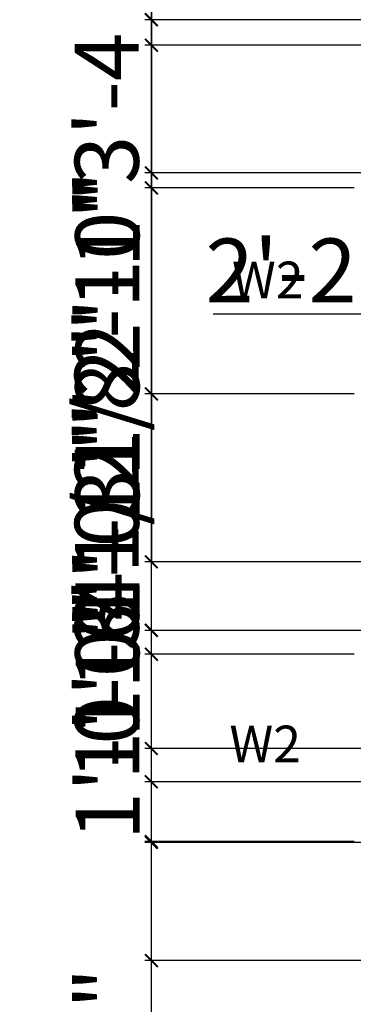
# Model space of a CAD drawing. Units: inches. Extents: x 1763 to 2368, y 1500 to 2097.
# Tile 5 of 24: x 1763 to 1828, y 1794 to 1986. Entities that reach past the tile are written whole.
import ezdxf

# ---------------------------------------------------------------- set-up
doc = ezdxf.new("R2010")
doc.units = ezdxf.units.IN
doc.layers.add('A-ANNO-DIMS', color=2, linetype='Continuous', lineweight=18)
doc.layers.add('A-ANNO-TEXT', color=7, linetype='Continuous', lineweight=18)
doc.styles.get("Standard").update_dxf_attribs({"font": 'arial.ttf'})
doc.dimstyles.new('ISO-25', dxfattribs={"dimtxt": 12.5, "dimasz": 2.5, "dimexe": 1.25, "dimexo": 0.625, "dimtad": 1, "dimdec": 0, "dimlunit": 4, "dimtxsty": 'Standard', "dimblk": 'ARCHTICK', "dimcen": 2.5, "dimclrd": 3, "dimclrt": 4, "dimadec": 0, "dimazin": 0, "dimtfac": 1, "dimtdec": 0, "dimtmove": 0, "dimatfit": 3, "dimfxl": 1, "dimarcsym": 0})

# ---------------------------------------------------------------- blocks, each defined once
blk = doc.blocks.new('_ArchTick')
at = {"color": 0, "linetype": 'ByBlock', "const_width": 0.15}
blk.add_lwpolyline([(-0.5, -0.5), (0.5, 0.5)], dxfattribs=at)
blk = doc.blocks.new('*D30')
at = {"layer": 'A-ANNO-DIMS', "color": 0, "lineweight": -2, "transparency": 16777216}
for p, q in [((1838.09, 1924.84), (1838.09, 1929.96)), ((1864.09, 1924.84), (1864.09, 1929.96))]:
    blk.add_line(p, q, dxfattribs=at)
at = {"layer": 'A-ANNO-DIMS', "color": 3, "lineweight": -2, "transparency": 16777216}
for p, q in [((1838.09, 1928.71), (1800.9, 1928.71)), ((1864.09, 1928.71), (1838.09, 1928.71))]:
    blk.add_line(p, q, dxfattribs=at)
at = {"layer": 'Defpoints', "color": 0, "transparency": 16777216}
for p in [(1838.09, 1928.71), (1838.09, 1924.21), (1864.09, 1924.21)]:
    blk.add_point(p, dxfattribs=at)
at = {"layer": 'A-ANNO-DIMS', "color": 3, "lineweight": -2, "transparency": 16777216, "xscale": 2.5, "yscale": 2.5, "zscale": 2.5, "rotation": 180}
blk.add_blockref('_ArchTick', (1838.09, 1928.71), dxfattribs=at)
at = {"layer": 'A-ANNO-DIMS', "color": 3, "lineweight": -2, "transparency": 16777216, "xscale": 2.5, "yscale": 2.5, "zscale": 2.5}
blk.add_blockref('_ArchTick', (1864.09, 1928.71), dxfattribs=at)
at = {"layer": 'A-ANNO-DIMS', "color": 4, "transparency": 16777216, "insert": (1818.25, 1935.61), "char_height": 12.5, "attachment_point": 5}
blk.add_mtext('2\'-2"', dxfattribs=at)
blk = doc.blocks.new('*D44')
at = {"layer": 'A-ANNO-DIMS', "color": 0, "lineweight": -2, "transparency": 16777216}
for p, q in [((1828.47, 2043.27), (1787.6, 2043.27)), ((1837.47, 1986.27), (1787.6, 1986.27))]:
    blk.add_line(p, q, dxfattribs=at)
at = {"layer": 'A-ANNO-DIMS', "color": 3, "lineweight": -2, "transparency": 16777216}
blk.add_line((1788.85, 2043.27), (1788.85, 1986.27), dxfattribs=at)
at = {"layer": 'Defpoints', "color": 0, "transparency": 16777216}
for p in [(1829.09, 2043.27), (1788.85, 1986.27), (1838.09, 1986.27)]:
    blk.add_point(p, dxfattribs=at)
at = {"layer": 'A-ANNO-DIMS', "color": 3, "lineweight": -2, "transparency": 16777216, "xscale": 2.5, "yscale": 2.5, "zscale": 2.5}
for p, rotation in [((1788.85, 2043.27), 90), ((1788.85, 1986.27), 270)]:
    blk.add_blockref('_ArchTick', p, dxfattribs=dict(at, rotation=rotation))
at = {"layer": 'A-ANNO-DIMS', "color": 4, "transparency": 16777216, "insert": (1781.85, 2014.77), "char_height": 12.5, "attachment_point": 5, "rotation": 90}
blk.add_mtext('4\'-9"', dxfattribs=at)
blk = doc.blocks.new('*D47')
at = {"layer": 'A-ANNO-DIMS', "color": 0, "lineweight": -2, "transparency": 16777216}
for p, q in [((1828.47, 1825.59), (1787.6, 1825.59)), ((1828.47, 1738.64), (1787.6, 1738.64))]:
    blk.add_line(p, q, dxfattribs=at)
at = {"layer": 'A-ANNO-DIMS', "color": 3, "lineweight": -2, "transparency": 16777216}
blk.add_line((1788.85, 1738.64), (1788.85, 1825.59), dxfattribs=at)
at = {"layer": 'Defpoints', "color": 0, "transparency": 16777216}
for p in [(1788.85, 1825.59), (1829.09, 1825.59), (1829.09, 1738.64)]:
    blk.add_point(p, dxfattribs=at)
at = {"layer": 'A-ANNO-DIMS', "color": 3, "lineweight": -2, "transparency": 16777216, "xscale": 2.5, "yscale": 2.5, "zscale": 2.5}
for p, rotation in [((1788.85, 1825.59), 90), ((1788.85, 1738.64), 270)]:
    blk.add_blockref('_ArchTick', p, dxfattribs=dict(at, rotation=rotation))
at = {"layer": 'A-ANNO-DIMS', "color": 4, "transparency": 16777216, "insert": (1781.84, 1782.12), "char_height": 12.5, "attachment_point": 5, "rotation": 90}
blk.add_mtext('7\'-3"', dxfattribs=at)
blk = doc.blocks.new('*D48')
at = {"layer": 'A-ANNO-DIMS', "color": 3, "lineweight": -2, "transparency": 16777216}
for p, q in [((1788.85, 1862.2), (1788.85, 1928.3)), ((1788.85, 1825.59), (1788.85, 1862.2))]:
    blk.add_line(p, q, dxfattribs=at)
at = {"layer": 'A-ANNO-DIMS', "color": 0, "lineweight": -2, "transparency": 16777216}
for p, q in [((1828.47, 1862.2), (1787.6, 1862.2)), ((1828.47, 1825.59), (1787.6, 1825.59))]:
    blk.add_line(p, q, dxfattribs=at)
at = {"layer": 'Defpoints', "color": 0, "transparency": 16777216}
for p in [(1788.85, 1862.2), (1829.09, 1862.2), (1829.09, 1825.59)]:
    blk.add_point(p, dxfattribs=at)
at = {"layer": 'A-ANNO-DIMS', "color": 3, "lineweight": -2, "transparency": 16777216, "xscale": 2.5, "yscale": 2.5, "zscale": 2.5}
for p, rotation in [((1788.85, 1862.2), 90), ((1788.85, 1825.59), 270)]:
    blk.add_blockref('_ArchTick', p, dxfattribs=dict(at, rotation=rotation))
at = {"layer": 'A-ANNO-DIMS', "color": 4, "transparency": 16777216, "insert": (1781.76, 1896.5), "char_height": 12.5, "attachment_point": 5, "rotation": 90}
blk.add_mtext('3\'-0 1/2"', dxfattribs=at)
blk = doc.blocks.new('*D49')
at = {"layer": 'A-ANNO-DIMS', "color": 0, "lineweight": -2, "transparency": 16777216}
for p, q in [((1828.47, 1913.1), (1787.6, 1913.1)), ((1828.47, 1862.2), (1787.6, 1862.2))]:
    blk.add_line(p, q, dxfattribs=at)
at = {"layer": 'A-ANNO-DIMS', "color": 3, "lineweight": -2, "transparency": 16777216}
blk.add_line((1788.85, 1862.2), (1788.85, 1913.1), dxfattribs=at)
at = {"layer": 'Defpoints', "color": 0, "transparency": 16777216}
for p in [(1788.85, 1913.1), (1829.09, 1913.1), (1829.09, 1862.2)]:
    blk.add_point(p, dxfattribs=at)
at = {"layer": 'A-ANNO-DIMS', "color": 3, "lineweight": -2, "transparency": 16777216, "xscale": 2.5, "yscale": 2.5, "zscale": 2.5}
for p, rotation in [((1788.85, 1913.1), 90), ((1788.85, 1862.2), 270)]:
    blk.add_blockref('_ArchTick', p, dxfattribs=dict(at, rotation=rotation))
at = {"layer": 'A-ANNO-DIMS', "color": 4, "transparency": 16777216, "insert": (1781.84, 1887.65), "char_height": 12.5, "attachment_point": 5, "rotation": 90}
blk.add_mtext('4\'-3"', dxfattribs=at)
blk = doc.blocks.new('*D50')
at = {"layer": 'A-ANNO-DIMS', "color": 3, "lineweight": -2, "transparency": 16777216}
for p, q in [((1788.85, 1953.39), (1788.85, 2019.48)), ((1788.85, 1913.1), (1788.85, 1953.39))]:
    blk.add_line(p, q, dxfattribs=at)
at = {"layer": 'A-ANNO-DIMS', "color": 0, "lineweight": -2, "transparency": 16777216}
for p, q in [((1828.47, 1953.39), (1787.6, 1953.39)), ((1828.47, 1913.1), (1787.6, 1913.1))]:
    blk.add_line(p, q, dxfattribs=at)
at = {"layer": 'Defpoints', "color": 0, "transparency": 16777216}
for p in [(1788.85, 1953.39), (1829.09, 1953.39), (1829.09, 1913.1)]:
    blk.add_point(p, dxfattribs=at)
at = {"layer": 'A-ANNO-DIMS', "color": 3, "lineweight": -2, "transparency": 16777216, "xscale": 2.5, "yscale": 2.5, "zscale": 2.5}
for p, rotation in [((1788.85, 1953.39), 90), ((1788.85, 1913.1), 270)]:
    blk.add_blockref('_ArchTick', p, dxfattribs=dict(at, rotation=rotation))
at = {"layer": 'A-ANNO-DIMS', "color": 4, "transparency": 16777216, "insert": (1781.76, 1987.69), "char_height": 12.5, "attachment_point": 5, "rotation": 90}
blk.add_mtext('3\'-4 1/2"', dxfattribs=at)
blk = doc.blocks.new('*D51')
at = {"layer": 'A-ANNO-DIMS', "color": 3, "lineweight": -2, "transparency": 16777216}
for p, q in [((1788.85, 1986.27), (1788.85, 2023.46)), ((1788.85, 1953.39), (1788.85, 1986.27))]:
    blk.add_line(p, q, dxfattribs=at)
at = {"layer": 'A-ANNO-DIMS', "color": 0, "lineweight": -2, "transparency": 16777216}
for p, q in [((1837.47, 1986.27), (1787.6, 1986.27)), ((1828.47, 1953.39), (1787.6, 1953.39))]:
    blk.add_line(p, q, dxfattribs=at)
at = {"layer": 'Defpoints', "color": 0, "transparency": 16777216}
for p in [(1788.85, 1986.27), (1838.09, 1986.27), (1829.09, 1953.39)]:
    blk.add_point(p, dxfattribs=at)
at = {"layer": 'A-ANNO-DIMS', "color": 3, "lineweight": -2, "transparency": 16777216, "xscale": 2.5, "yscale": 2.5, "zscale": 2.5}
for p, rotation in [((1788.85, 1986.27), 90), ((1788.85, 1953.39), 270)]:
    blk.add_blockref('_ArchTick', p, dxfattribs=dict(at, rotation=rotation))
at = {"layer": 'A-ANNO-DIMS', "color": 4, "transparency": 16777216, "insert": (1781.85, 2006.12), "char_height": 12.5, "attachment_point": 5, "rotation": 90}
blk.add_mtext('2\'-9"', dxfattribs=at)
blk = doc.blocks.new('*D79')
at = {"layer": 'A-ANNO-DIMS', "color": 3, "lineweight": -2, "transparency": 16777216}
for p, q in [((1788.85, 1825.4), (1788.85, 1870.91)), ((1788.85, 1802.3), (1788.85, 1825.4))]:
    blk.add_line(p, q, dxfattribs=at)
at = {"layer": 'A-ANNO-DIMS', "color": 0, "lineweight": -2, "transparency": 16777216}
for p, q in [((2054.47, 1825.4), (1787.6, 1825.4)), ((2054.47, 1802.3), (1787.6, 1802.3))]:
    blk.add_line(p, q, dxfattribs=at)
at = {"layer": 'Defpoints', "color": 0, "transparency": 16777216}
for p in [(1788.85, 1825.4), (2055.09, 1825.4), (2055.09, 1802.3)]:
    blk.add_point(p, dxfattribs=at)
at = {"layer": 'A-ANNO-DIMS', "color": 3, "lineweight": -2, "transparency": 16777216, "xscale": 2.5, "yscale": 2.5, "zscale": 2.5}
for p, rotation in [((1788.85, 1825.4), 90), ((1788.85, 1802.3), 270)]:
    blk.add_blockref('_ArchTick', p, dxfattribs=dict(at, rotation=rotation))
at = {"layer": 'A-ANNO-DIMS', "color": 4, "transparency": 16777216, "insert": (1781.95, 1849.4), "char_height": 12.5, "attachment_point": 5, "rotation": 90}
blk.add_mtext('1\'-11"', dxfattribs=at)
blk = doc.blocks.new('*D80')
at = {"layer": 'A-ANNO-DIMS', "color": 3, "lineweight": -2, "transparency": 16777216}
for p, q in [((1788.85, 1837.27), (1788.85, 1873.07)), ((1788.85, 1825.4), (1788.85, 1837.27))]:
    blk.add_line(p, q, dxfattribs=at)
at = {"layer": 'A-ANNO-DIMS', "color": 0, "lineweight": -2, "transparency": 16777216}
for p, q in [((2054.47, 1837.27), (1787.6, 1837.27)), ((2054.47, 1825.4), (1787.6, 1825.4))]:
    blk.add_line(p, q, dxfattribs=at)
at = {"layer": 'Defpoints', "color": 0, "transparency": 16777216}
for p in [(1788.85, 1837.27), (2055.09, 1837.27), (2055.09, 1825.4)]:
    blk.add_point(p, dxfattribs=at)
at = {"layer": 'A-ANNO-DIMS', "color": 3, "lineweight": -2, "transparency": 16777216, "xscale": 2.5, "yscale": 2.5, "zscale": 2.5}
for p, rotation in [((1788.85, 1837.27), 90), ((1788.85, 1825.4), 270)]:
    blk.add_blockref('_ArchTick', p, dxfattribs=dict(at, rotation=rotation))
at = {"layer": 'A-ANNO-DIMS', "color": 4, "transparency": 16777216, "insert": (1781.85, 1856.42), "char_height": 12.5, "attachment_point": 5, "rotation": 90}
blk.add_mtext('1\'-0"', dxfattribs=at)
blk = doc.blocks.new('*D81')
at = {"layer": 'A-ANNO-DIMS', "color": 3, "lineweight": -2, "transparency": 16777216}
for p, q in [((1788.85, 1866.87), (1788.85, 1912.38)), ((1788.85, 1843.77), (1788.85, 1866.87))]:
    blk.add_line(p, q, dxfattribs=at)
at = {"layer": 'A-ANNO-DIMS', "color": 0, "lineweight": -2, "transparency": 16777216}
for p, q in [((2077.47, 1866.87), (1787.6, 1866.87)), ((2077.47, 1843.77), (1787.6, 1843.77))]:
    blk.add_line(p, q, dxfattribs=at)
at = {"layer": 'Defpoints', "color": 0, "transparency": 16777216}
for p in [(1788.85, 1866.87), (2078.09, 1866.87), (2078.09, 1843.77)]:
    blk.add_point(p, dxfattribs=at)
at = {"layer": 'A-ANNO-DIMS', "color": 3, "lineweight": -2, "transparency": 16777216, "xscale": 2.5, "yscale": 2.5, "zscale": 2.5}
for p, rotation in [((1788.85, 1866.87), 90), ((1788.85, 1843.77), 270)]:
    blk.add_blockref('_ArchTick', p, dxfattribs=dict(at, rotation=rotation))
at = {"layer": 'A-ANNO-DIMS', "color": 4, "transparency": 16777216, "insert": (1781.95, 1890.87), "char_height": 12.5, "attachment_point": 5, "rotation": 90}
blk.add_mtext('1\'-11"', dxfattribs=at)
blk = doc.blocks.new('*D82')
at = {"layer": 'A-ANNO-DIMS', "color": 3, "lineweight": -2, "transparency": 16777216}
for p, q in [((1788.85, 1843.77), (1788.85, 1909.87)), ((1788.85, 1837.27), (1788.85, 1843.77))]:
    blk.add_line(p, q, dxfattribs=at)
at = {"layer": 'A-ANNO-DIMS', "color": 0, "lineweight": -2, "transparency": 16777216}
for p, q in [((2077.47, 1843.77), (1787.6, 1843.77)), ((2077.47, 1837.27), (1787.6, 1837.27))]:
    blk.add_line(p, q, dxfattribs=at)
at = {"layer": 'Defpoints', "color": 0, "transparency": 16777216}
for p in [(1788.85, 1843.77), (2078.09, 1843.77), (2078.09, 1837.27)]:
    blk.add_point(p, dxfattribs=at)
at = {"layer": 'A-ANNO-DIMS', "color": 3, "lineweight": -2, "transparency": 16777216, "xscale": 2.5, "yscale": 2.5, "zscale": 2.5}
for p, rotation in [((1788.85, 1843.77), 90), ((1788.85, 1837.27), 270)]:
    blk.add_blockref('_ArchTick', p, dxfattribs=dict(at, rotation=rotation))
at = {"layer": 'A-ANNO-DIMS', "color": 4, "transparency": 16777216, "insert": (1781.77, 1878.07), "char_height": 12.5, "attachment_point": 5, "rotation": 90}
blk.add_mtext('0\'-6 1/2"', dxfattribs=at)
blk = doc.blocks.new('*D85')
at = {"layer": 'A-ANNO-DIMS', "color": 0, "lineweight": -2, "transparency": 16777216}
for p, q in [((1957.47, 1986.27), (1787.6, 1986.27)), ((1958.51, 1880.27), (1787.6, 1880.27))]:
    blk.add_line(p, q, dxfattribs=at)
at = {"layer": 'A-ANNO-DIMS', "color": 3, "lineweight": -2, "transparency": 16777216}
blk.add_line((1788.85, 1986.27), (1788.85, 1880.27), dxfattribs=at)
at = {"layer": 'Defpoints', "color": 0, "transparency": 16777216}
for p in [(1958.09, 1986.27), (1788.85, 1880.27), (1959.13, 1880.27)]:
    blk.add_point(p, dxfattribs=at)
at = {"layer": 'A-ANNO-DIMS', "color": 3, "lineweight": -2, "transparency": 16777216, "xscale": 2.5, "yscale": 2.5, "zscale": 2.5}
for p, rotation in [((1788.85, 1986.27), 90), ((1788.85, 1880.27), 270)]:
    blk.add_blockref('_ArchTick', p, dxfattribs=dict(at, rotation=rotation))
at = {"layer": 'A-ANNO-DIMS', "color": 4, "transparency": 16777216, "insert": (1781.85, 1933.27), "char_height": 12.5, "attachment_point": 5, "rotation": 90}
blk.add_mtext('8\'-10"', dxfattribs=at)
blk = doc.blocks.new('*D91')
at = {"layer": 'A-ANNO-DIMS', "color": 0, "lineweight": -2, "transparency": 16777216}
for p, q in [((1935.72, 1981.27), (1787.6, 1981.27)), ((1935.72, 1956.32), (1787.6, 1956.32))]:
    blk.add_line(p, q, dxfattribs=at)
at = {"layer": 'A-ANNO-DIMS', "color": 3, "lineweight": -2, "transparency": 16777216}
for p, q in [((1788.85, 1981.27), (1788.85, 1956.32)), ((1788.85, 1956.32), (1788.85, 1919.13))]:
    blk.add_line(p, q, dxfattribs=at)
at = {"layer": 'Defpoints', "color": 0, "transparency": 16777216}
for p in [(1936.34, 1981.27), (1788.85, 1956.32), (1936.34, 1956.32)]:
    blk.add_point(p, dxfattribs=at)
at = {"layer": 'A-ANNO-DIMS', "color": 3, "lineweight": -2, "transparency": 16777216, "xscale": 2.5, "yscale": 2.5, "zscale": 2.5}
for p, rotation in [((1788.85, 1981.27), 90), ((1788.85, 1956.32), 270)]:
    blk.add_blockref('_ArchTick', p, dxfattribs=dict(at, rotation=rotation))
at = {"layer": 'A-ANNO-DIMS', "color": 4, "transparency": 16777216, "insert": (1781.95, 1936.48), "char_height": 12.5, "attachment_point": 5, "rotation": 90}
blk.add_mtext('2\'-1"', dxfattribs=at)

msp = doc.modelspace()

# ---------------------------------------------------------------- texts
at = {"layer": 'A-ANNO-TEXT'}
for p in [(1804.6, 1931.82), (1804.1, 1841.09)]:
    msp.add_text('W2', height=7.155, dxfattribs=at).set_placement(p)

# ---------------------------------------------------------------- dimensions: what is measured, and where the dimension line sits
at = {"layer": 'A-ANNO-DIMS'}
for base, p1, p2, angle, picture, middle in [((1788.85, 1986.27), (1829.09, 2043.27), (1838.09, 1986.27), 90, '*D44', (1781.85, 2014.77)), ((1788.85, 1986.27), (1829.09, 1953.39), (1838.09, 1986.27), 90, '*D51', (1781.85, 2006.12)), ((1788.85, 1953.39), (1829.09, 1913.1), (1829.09, 1953.39), 90, '*D50', (1781.76, 1987.69)), ((1788.85, 1880.27), (1958.09, 1986.27), (1959.13, 1880.27), 90, '*D85', (1781.85, 1933.27)), ((1788.8549, 1956.3234), (1936.3405, 1981.2727), (1936.3405, 1956.3234), 90, '*D91', (1781.9543, 1936.4778)), ((1838.09, 1928.71), (1864.09, 1924.21), (1838.09, 1924.21), 180, '*D30', (1818.25, 1935.61)), ((1788.85, 1862.2), (1829.09, 1825.59), (1829.09, 1862.2), 90, '*D48', (1781.76, 1896.5)), ((1788.85, 1913.1), (1829.09, 1862.2), (1829.09, 1913.1), 90, '*D49', (1781.84, 1887.65)), ((1788.85, 1866.87), (2078.09, 1843.77), (2078.09, 1866.87), 90, '*D81', (1781.95, 1890.87)), ((1788.85, 1843.77), (2078.09, 1837.27), (2078.09, 1843.77), 90, '*D82', (1781.77, 1878.07)), ((1788.85, 1837.27), (2055.09, 1825.4), (2055.09, 1837.27), 90, '*D80', (1781.85, 1856.42)), ((1788.85, 1825.4), (2055.09, 1802.3), (2055.09, 1825.4), 90, '*D79', (1781.95, 1849.4)), ((1788.8549, 1825.5896), (1829.0918, 1738.6434), (1829.0918, 1825.5896), 90, '*D47', (1781.8435, 1782.1165))]:
    dim = msp.add_linear_dim(base=base, p1=p1, p2=p2, angle=angle, dimstyle='ISO-25', override={"dimdec": 1, "dimlfac": 1, "dimrnd": 0, "dimzin": 1, "dimdsep": 46, "dimlunit": 4, "dimfrac": 2}, dxfattribs=at)
    dim.commit()
    dim.dimension.update_dxf_attribs({"geometry": picture, "text_midpoint": middle})

doc.saveas('drawing.dxf')
